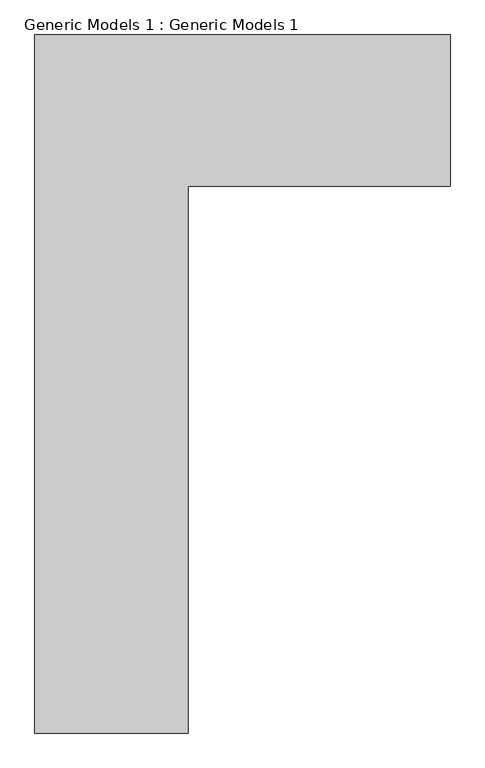
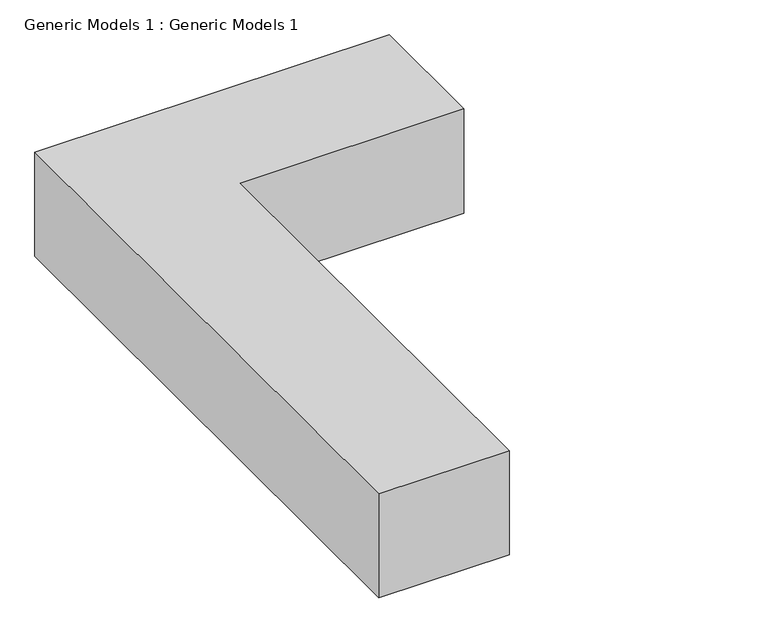
"""IFC4 building model written with IfcOpenShell, lengths in millimetres: proxy geometry, Generic Models 1 : Generic Models 1."""

from ifc_helpers import new_model, si_unit, origin, origin_with_axes, place, context, project, spatial, polyline, outline, extrude, source, transform, mapped, element, save


def generic_models_1_generic_models_1_540f675e(model_context):
    return source(origin(), model_context, "Body", "SweptSolid", [
        extrude(outline(polyline([(-5793.4988863, 5000.2647258), (-6860.2988863, 5000.2647258), (-6860.2988863, 9864.3647258), (-3964.6988863, 9864.3647258), (-3964.6988863, 8810.2647258), (-5793.4988863, 8810.2647258), (-5793.4988863, 5000.2647258)])), origin_with_axes(), (0.0, 0.0, 1.0), 900.0),
    ])


if __name__ == "__main__":
    model = new_model("IFC4")
    model_context = context("Model", 3, world=origin())
    ifc_project = project(units=[si_unit("LENGTHUNIT", "METRE", prefix="MILLI")], contexts=[model_context])
    site = spatial("IfcSite", under=ifc_project)
    building = spatial("IfcBuilding", under=site)
    placement = place(None, origin())
    generic_models_1_generic_models_1_shape = generic_models_1_generic_models_1_540f675e(model_context)
    element("IfcBuildingElementProxy", 1, Name="Generic Models 1 : Generic Models 1", ObjectType="Generic Models 1 : Generic Models 1", at=placement, inside=building, context=model_context, shape_type="MappedRepresentation", body=[
        mapped(generic_models_1_generic_models_1_shape, transform((0.0, 0.0, 0.0), x_axis=(1.0, 0.0, 0.0), y_axis=(0.0, 1.0, 0.0), z_axis=(0.0, 0.0, 1.0))),
    ])
    save(model, "model.ifc")
